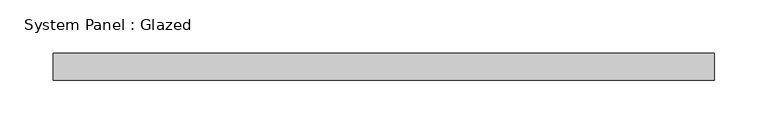
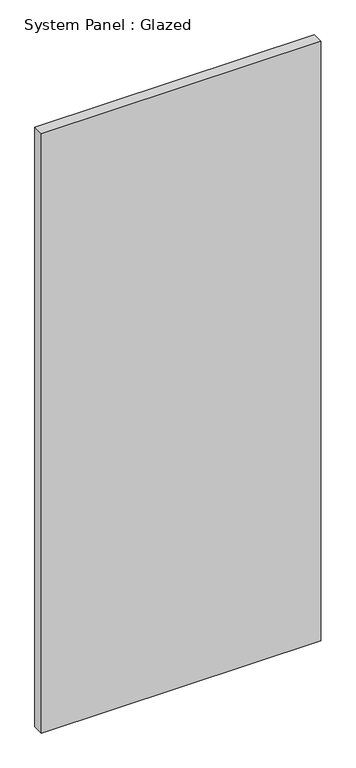
"""IFC4 building model written with IfcOpenShell, lengths in millimetres: plate geometry, System Panel : Glazed."""

from ifc_helpers import new_model, si_unit, origin, origin_with_axes, place, context, project, spatial, polyline, outline, extrude, source, transform, mapped, element, save


def system_panel_glazed_b7a4a9c9(model_context):
    return source(origin(), model_context, "Body", "SweptSolid", [
        extrude(outline(polyline([(311.15, 19.05), (-311.15, 19.05), (-311.15, 44.45), (311.15, 44.45), (311.15, 19.05)])), origin_with_axes(), (0.0, 0.0, 1.0), 1412.437083),
    ])


if __name__ == "__main__":
    model = new_model("IFC4")
    model_context = context("Model", 3, world=origin())
    ifc_project = project(units=[si_unit("LENGTHUNIT", "METRE", prefix="MILLI")], contexts=[model_context])
    site = spatial("IfcSite", under=ifc_project)
    building = spatial("IfcBuilding", under=site)
    placement = place(None, origin())
    system_panel_glazed_shape = system_panel_glazed_b7a4a9c9(model_context)
    element("IfcPlate", 1, ObjectType="System Panel : Glazed", at=placement, inside=building, context=model_context, shape_type="MappedRepresentation", body=[
        mapped(system_panel_glazed_shape, transform((0.0, 0.0, 0.0), x_axis=(1.0, 0.0, 0.0), y_axis=(0.0, 1.0, 0.0), z_axis=(0.0, 0.0, 1.0))),
    ])
    save(model, "model.ifc")

# Revit data of these elements
# Type "System Panel : Glazed"
#   Construction Type Id = "GSP4R"
#   Analytic Construction = "1/8 in Pilkington single glazing"
#   Visual Light Transmittance = 0.9
#   Solar Heat Gain Coefficient = 0.86
#   Heat Transfer Coefficient (U) = 1.18115 BTU/(h·ft²·°F)
#   Define Thermal Properties by = 1
# Element 1 (IfcPlate, "System Panel : Glazed")
#   Materials on its faces: "Glass"
# Materials
#   "Glass": class "Glass", colour RGB 0 128 192, transparency 0.75, Description = "Soda Lime Glass", Cost = 0
